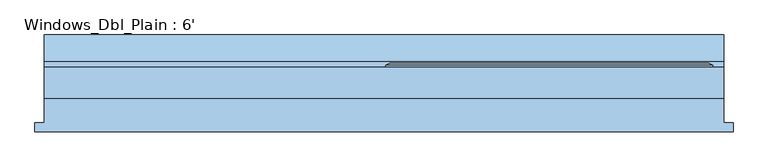
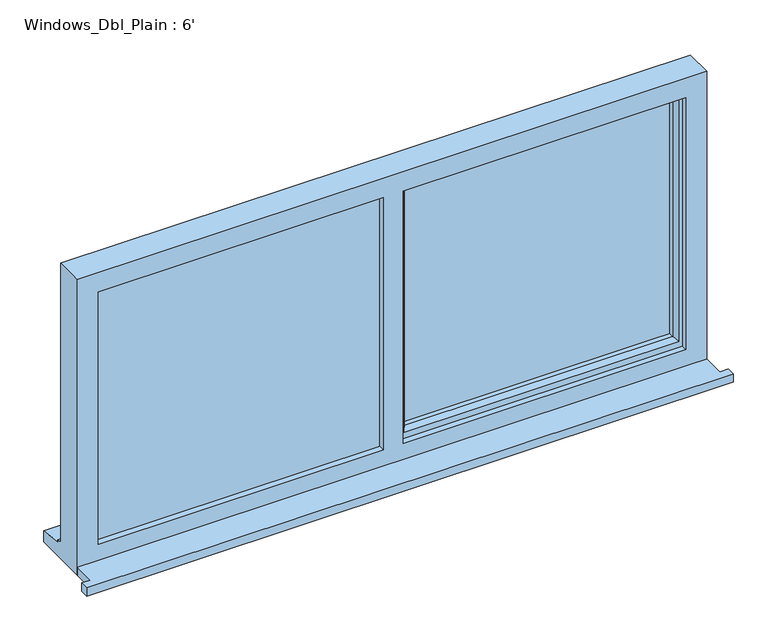
"""IFC4 building model written with IfcOpenShell, lengths in millimetres: window geometry, Windows_Dbl_Plain : 6'."""

from ifc_helpers import new_model, si_unit, frame, origin, place, context, project, spatial, polyline, outline, extrude, faceted_brep, source, transform, mapped, element, save


def windows_dbl_plain_6_decf5736(model_context):
    return source(origin(), model_context, "Body", "SolidModel", [
        extrude(outline(polyline([(-1224.4, -115.6034322), (-1224.4, -90.6034322), (-1199.4, -90.6034322), (-1199.4, -25.4834322), (629.4, -25.4834322), (629.4, -90.6034322), (654.4, -90.6034322), (654.4, -115.6034322), (-1224.4, -115.6034322)])), frame((0.0, 0.0, 1200.0), z_axis=(0.0, 0.0, 1.0), x_axis=(1.0, 0.0, 0.0)), (0.0, 0.0, 1.0), 25.0),
        faceted_brep([(-280.0, 57.5165678, 2080.0), (-280.0, 63.2900705, 2080.0), (-280.0, 63.2900705, 1253.0), (-280.0, 57.5165678, 1253.0), (-270.0, -7.4834322, 2070.0), (-270.0, 57.5165678, 2070.0), (-270.0, 57.5165678, 1263.0), (-270.0, -7.4834322, 1263.0), (-230.0, 7.0094677, 2030.0), (-240.1480377, -7.4834322, 2040.1480377), (-240.1480377, -7.4834322, 1292.8519623), (-230.0, 7.0094677, 1303.0), (-230.0, 21.5165678, 2030.0), (-230.0, 21.5165678, 1303.0), (-240.0, 45.5165678, 2040.0), (-240.0, 21.5165678, 2040.0), (-240.0, 21.5165678, 1293.0), (-240.0, 45.5165678, 1293.0), (-230.0, 63.2900705, 2030.0), (-230.0, 45.5165678, 2030.0), (-230.0, 45.5165678, 1303.0), (-230.0, 63.2900705, 1303.0), (-247.4457548, 69.0635732, 2047.4457548), (-247.4457548, 69.0635732, 1285.5542452), (-269.2153903, 69.0635732, 2069.2153903), (-269.2153903, 69.0635732, 1263.7846097), (599.4, 63.2900705, 1253.0), (599.4, 57.5165678, 1253.0), (589.4, 57.5165678, 1263.0), (589.4, -7.4834322, 1263.0), (559.5480377, -7.4834322, 1292.8519623), (549.4, 7.0094677, 1303.0), (549.4, 21.5165678, 1303.0), (559.4, 21.5165678, 1293.0), (559.4, 45.5165678, 1293.0), (549.4, 45.5165678, 1303.0), (549.4, 63.2900705, 1303.0), (566.8457548, 69.0635732, 1285.5542452), (588.6153903, 69.0635732, 1263.7846097), (599.4, 63.2900705, 2080.0), (599.4, 57.5165678, 2080.0), (589.4, 57.5165678, 2070.0), (589.4, -7.4834322, 2070.0), (559.5480377, -7.4834322, 2040.1480377), (549.4, 7.0094677, 2030.0), (549.4, 21.5165678, 2030.0), (559.4, 21.5165678, 2040.0), (559.4, 45.5165678, 2040.0), (549.4, 45.5165678, 2030.0), (549.4, 63.2900705, 2030.0), (566.8457548, 69.0635732, 2047.4457548), (588.6153903, 69.0635732, 2069.2153903)], [[[0, 1, 2, 3]], [[4, 5, 6, 7]], [[8, 9, 10, 11]], [[12, 8, 11, 13]], [[14, 15, 16, 17]], [[18, 19, 20, 21]], [[22, 18, 21, 23]], [[1, 24, 25, 2]], [[3, 2, 26, 27]], [[7, 6, 28, 29]], [[11, 10, 30, 31]], [[13, 11, 31, 32]], [[17, 16, 33, 34]], [[21, 20, 35, 36]], [[23, 21, 36, 37]], [[2, 25, 38, 26]], [[27, 26, 39, 40]], [[29, 28, 41, 42]], [[31, 30, 43, 44]], [[32, 31, 44, 45]], [[34, 33, 46, 47]], [[36, 35, 48, 49]], [[37, 36, 49, 50]], [[26, 38, 51, 39]], [[40, 39, 1, 0]], [[3, 27, 40, 0], [5, 41, 28, 6]], [[42, 41, 5, 4]], [[7, 29, 42, 4], [9, 43, 30, 10]], [[44, 43, 9, 8]], [[45, 44, 8, 12]], [[15, 46, 33, 16], [13, 32, 45, 12]], [[47, 46, 15, 14]], [[17, 34, 47, 14], [19, 48, 35, 20]], [[49, 48, 19, 18]], [[50, 49, 18, 22]], [[24, 51, 38, 25], [23, 37, 50, 22]], [[39, 51, 24, 1]]]),
        extrude(outline(polyline([(2050.0, -310.0), (2070.0, -310.0), (2070.0, -1159.4), (1263.0, -1159.4), (1263.0, -310.0), (1283.0, -310.0), (1283.0, -1139.4), (2050.0, -1139.4), (2050.0, -310.0)])), frame((0.0, 16.5165678, 0.0), z_axis=(0.0, 1.0, 0.0), x_axis=(0.0, 0.0, 1.0)), (0.0, 0.0, 1.0), 41.0),
        faceted_brep([(629.4, -25.4834322, 2110.0), (-1199.4, -25.4834322, 2110.0), (-1199.4, -25.4834322, 1200.0), (629.4, -25.4834322, 1200.0), (569.4, -25.4834322, 2050.0), (569.4, -25.4834322, 1275.0), (-252.0, -25.4834322, 1275.0), (-252.0, -25.4834322, 2050.0), (-310.0, -25.4834322, 2050.0), (-310.0, -25.4834322, 1275.0), (-1139.4, -25.4834322, 1275.0), (-1139.4, -25.4834322, 2050.0), (-1199.4, 57.5165678, 2110.0), (-1199.4, 57.5165678, 1251.0), (-1199.4, 72.5165678, 1249.68767), (-1199.4, 72.5165678, 1244.7449676), (-1199.4, 145.0165678, 1233.8088847), (-1199.4, 145.0165678, 1200.0), (629.4, 57.5165678, 2110.0), (629.4, 57.5165678, 1251.0), (-1159.4, 57.5165678, 2070.0), (-1159.4, 57.5165678, 1263.0), (-310.0, 57.5165678, 1263.0), (-310.0, 57.5165678, 2070.0), (-270.0, 57.5165678, 2070.0), (-270.0, 57.5165678, 1263.0), (589.4, 57.5165678, 1263.0), (589.4, 57.5165678, 2070.0), (-1159.4, -7.4834322, 2070.0), (-1159.4, -7.4834322, 1263.0), (-300.0, -7.4834322, 2070.0), (-300.0, -7.4834322, 1263.0), (-310.0, -7.4834322, 2050.0), (-1139.4, -7.4834322, 2050.0), (-1139.4, -7.4834322, 1275.0), (-310.0, -7.4834322, 1275.0), (-270.0, -7.4834322, 2070.0), (589.4, -7.4834322, 2070.0), (589.4, -7.4834322, 1263.0), (-270.0, -7.4834322, 1263.0), (569.4, -7.4834322, 2050.0), (-252.0, -7.4834322, 2050.0), (-252.0, -7.4834322, 1275.0), (569.4, -7.4834322, 1275.0), (-310.0, 16.5165678, 2070.0), (-300.0, 16.5165678, 2070.0), (629.4, 145.0165678, 1200.0), (629.4, 145.0165678, 1233.8088847), (629.4, 72.5165678, 1244.7449676), (629.4, 72.5165678, 1249.68767), (-300.0, 16.5165678, 1263.0), (-310.0, 16.5165678, 1263.0)], [[[0, 1, 2, 3], [4, 5, 6, 7], [8, 9, 10, 11]], [[2, 1, 12, 13, 14, 15, 16, 17]], [[13, 12, 18, 19], [20, 21, 22, 23], [24, 25, 26, 27]], [[21, 20, 28, 29]], [[28, 30, 31, 29], [32, 33, 34, 35]], [[36, 37, 38, 39], [40, 41, 42, 43]], [[33, 11, 10, 34]], [[1, 0, 18, 12]], [[28, 20, 23, 44, 45, 30]], [[27, 37, 36, 24]], [[11, 33, 32, 8]], [[40, 4, 7, 41]], [[19, 18, 0, 3, 46, 47, 48, 49]], [[27, 26, 38, 37]], [[4, 40, 43, 5]], [[45, 50, 31, 30]], [[50, 45, 44, 51]], [[51, 44, 23, 22]], [[25, 24, 36, 39]], [[41, 7, 6, 42]], [[8, 32, 35, 9]], [[46, 3, 2, 17]], [[47, 46, 17, 16]], [[48, 47, 16, 15]], [[49, 48, 15, 14]], [[19, 49, 14, 13]], [[22, 21, 29, 31, 50, 51]], [[26, 25, 39, 38]], [[6, 5, 43, 42]], [[35, 34, 10, 9]]]),
        extrude(outline(polyline([(-1159.4, 16.5165678), (-300.0, 16.5165678), (-300.0, -7.4834322), (-1159.4, -7.4834322), (-1159.4, 16.5165678)])), frame((0.0, 0.0, 1263.0), z_axis=(0.0, 0.0, 1.0), x_axis=(1.0, 0.0, 0.0)), (0.0, 0.0, 1.0), 807.0),
        extrude(outline(polyline([(559.4, 21.5165678), (-240.0, 21.5165678), (-240.0, 45.5165678), (559.4, 45.5165678), (559.4, 21.5165678)])), frame((0.0, 0.0, 1293.0), z_axis=(0.0, 0.0, 1.0), x_axis=(1.0, 0.0, 0.0)), (0.0, 0.0, 1.0), 747.0),
    ])


if __name__ == "__main__":
    model = new_model("IFC4")
    model_context = context("Model", 3, world=origin())
    ifc_project = project(units=[si_unit("LENGTHUNIT", "METRE", prefix="MILLI")], contexts=[model_context])
    site = spatial("IfcSite", under=ifc_project)
    building = spatial("IfcBuilding", under=site)
    placement = place(None, origin())
    windows_dbl_plain_6_shape = windows_dbl_plain_6_decf5736(model_context)
    element("IfcWindow", 1, ObjectType="Windows_Dbl_Plain : 6'", at=placement, inside=building, context=model_context, shape_type="MappedRepresentation", body=[
        mapped(windows_dbl_plain_6_shape, transform((0.0, 0.0, 0.0), x_axis=(1.0, 0.0, 0.0), y_axis=(0.0, 1.0, 0.0), z_axis=(0.0, 0.0, 1.0))),
    ])
    save(model, "model.ifc")

# Revit data of these elements
# Type "Windows_Dbl_Plain : 6'"
#   Type Mark = "62"
#   Operation = "DoublePanelVertical"
#   Construction Type Id = "GSP4R"
#   Manufacturer = "Revit"
#   Keynote = "L10"
#   Analytic Construction = "1/8 in Pilkington single glazing"
#   Wrap Layers (Ext) from Ext = 0.336286 ft
#   Wrap Layers (Int) from Ext = 0.582349 ft
#   Window Board Projection = 0.082021 ft
#   Window Board Extension = 0.082021 ft
#   Visual Light Transmittance = 0.9
#   Solar Heat Gain Coefficient = 0.78
#   Rough Width = 6.0 ft
#   Rough Height = 2.985564 ft
#   Height = 2.985564 ft
#   Width = 6.0 ft
#   Heat Transfer Coefficient (U) = 3.6886 W/(m²·K)
#   Glazing Thickness = 0.07874 ft
#   FrameOffset - External = 0.164042 ft
#   Frame Depth = 0.213255 ft
#   Default Head Height = 6.922572 ft
#   Cill Depth = 0.287073 ft
#   Cavity Closer Width = 0.164042 ft
#   Cavity Closer Offset from Ext = 0.336286 ft
#   Cavity Closer Depth = 0.278871 ft
#   Vis - Cavity Closers = yes
#   Define Thermal Properties by = 1
#   Material Trim = Window Frame
#   Material Glass = Glass
#   Material Frame = Window Frame
#   Wall Closure = (empty or 0)
# Element 1 (IfcWindow, "Windows_Dbl_Plain : 6'")
#   Materials on its faces: "Window Frame", "Glass"
# Materials
#   "Window Frame": colour RGB 249 249 249, transparency 0, Keynote = "L10", Cost = 0
#   "Glass": class "Glass", colour RGB 0 128 192, transparency 0.9, Description = "Soda Lime Glass", Cost = 0
